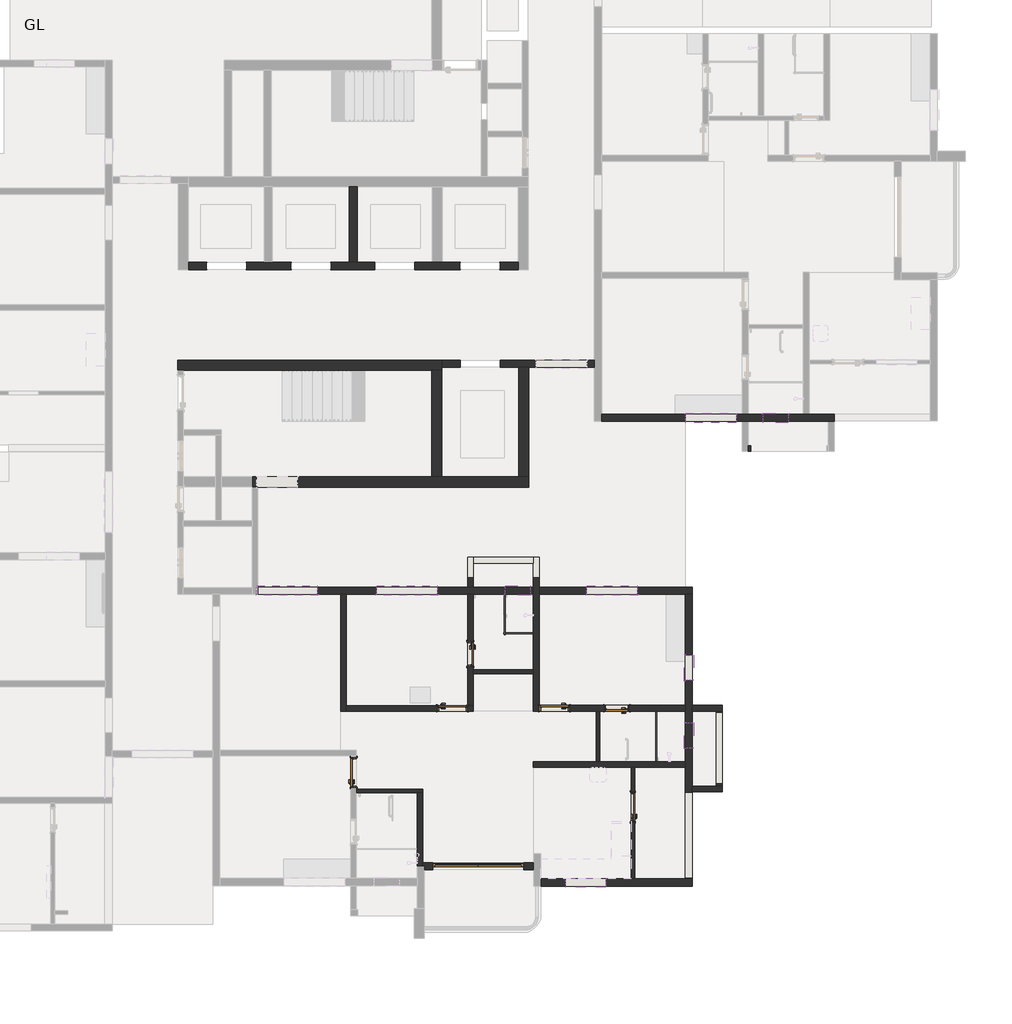
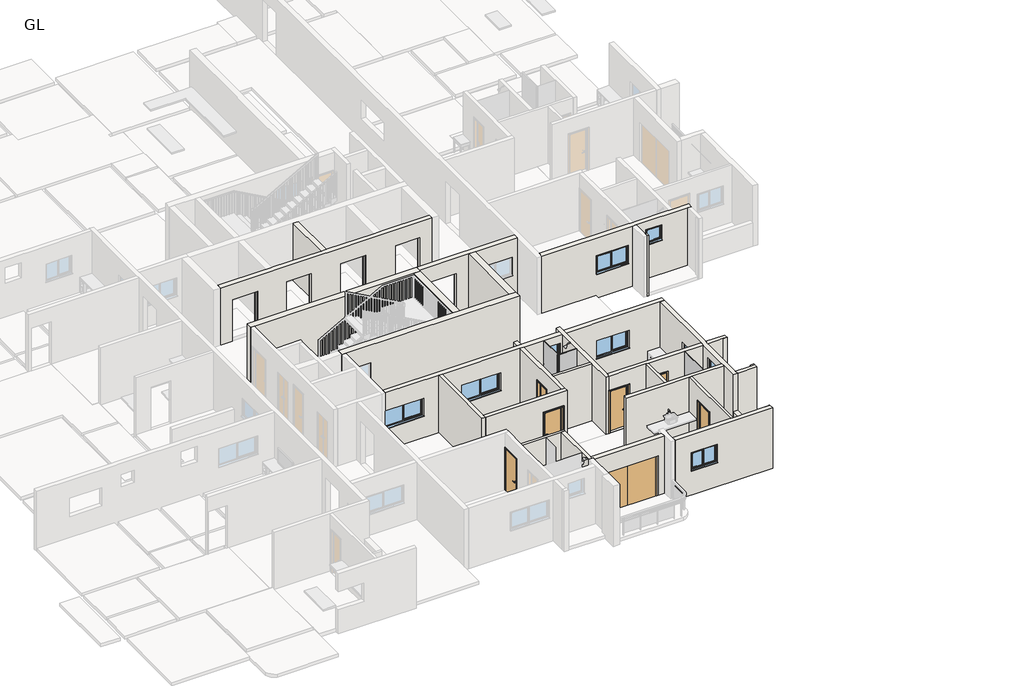
# One storey, part 4 of 14: 35 walls, 9 windows, 7 doors, 3 plates.
# Revit data of these elements (continued)
# Type "Windows_Dbl_Plain : 5'" (continued)
#   Rough Width = 5.0 ft
#   Rough Height = 2.985564 ft
#   Height = 2.985564 ft
#   Width = 5.0 ft
#   Heat Transfer Coefficient (U) = 3.6886 W/(m²·K)
#   Glazing Thickness = 0.07874 ft
#   FrameOffset - External = 0.164042 ft
#   Frame Depth = 0.213255 ft
#   Default Head Height = 6.922572 ft
#   Cill Depth = 0.287073 ft
#   Cavity Closer Width = 0.164042 ft
#   Cavity Closer Offset from Ext = 0.336286 ft
#   Cavity Closer Depth = 0.278871 ft
#   Vis - Cavity Closers = yes
#   Define Thermal Properties by = 1
#   Material Trim = Window Frame
#   Material Glass = Glass
#   Material Frame = Window Frame
#   Wall Closure = (empty or 0)
# Type "Windows_Dbl_Plain : 6'"
#   Type Mark = "62"
#   Operation = "DoublePanelVertical"
#   Construction Type Id = "GSP4R"
#   Manufacturer = "Revit"
#   Keynote = "L10"
#   Analytic Construction = "1/8 in Pilkington single glazing"
#   Wrap Layers (Ext) from Ext = 0.336286 ft
#   Wrap Layers (Int) from Ext = 0.582349 ft
#   Window Board Projection = 0.082021 ft
#   Window Board Extension = 0.082021 ft
#   Visual Light Transmittance = 0.9
#   Solar Heat Gain Coefficient = 0.78
#   Rough Width = 6.0 ft
#   Rough Height = 2.985564 ft
#   Height = 2.985564 ft
#   Width = 6.0 ft
#   Heat Transfer Coefficient (U) = 3.6886 W/(m²·K)
#   Glazing Thickness = 0.07874 ft
#   FrameOffset - External = 0.164042 ft
#   Frame Depth = 0.213255 ft
#   Default Head Height = 6.922572 ft
#   Cill Depth = 0.287073 ft
#   Cavity Closer Width = 0.164042 ft
#   Cavity Closer Offset from Ext = 0.336286 ft
#   Cavity Closer Depth = 0.278871 ft
#   Vis - Cavity Closers = yes
#   Define Thermal Properties by = 1
#   Material Trim = Window Frame
#   Material Glass = Glass
#   Material Frame = Window Frame
#   Wall Closure = (empty or 0)
# Type "Windows_Sgl_Plain : 2.5'"
#   Type Mark = "61"
#   Operation = "SinglePanel"
#   Construction Type Id = "SGL"
#   Manufacturer = "Revit"
#   Keynote = "L10"
#   Analytic Construction = "Large single-glazed windows"
#   Wrap Layers (Ext) from Ext = 0.336286 ft
#   Wrap Layers (Int) from Ext = 0.582349 ft
#   Window Board Projection = 0.082021 ft
#   Window Board Extension = 0.082021 ft
#   Visual Light Transmittance = 0.9
#   Solar Heat Gain Coefficient = 0.86
#   Rough Width = 2.5 ft
#   Rough Height = 2.5 ft
#   Height = 2.5 ft
#   Width = 2.5 ft
#   Heat Transfer Coefficient (U) = 5.5617 W/(m²·K)
#   Glazing Thickness = 0.07874 ft
#   FrameOffset - External = 0.164042 ft
#   Frame Depth = 0.213255 ft
#   Default Head Height = 6.922572 ft
#   Cill Depth = 0.287073 ft
#   Cavity Closer Width = 0.164042 ft
#   Cavity Closer Offset from Ext = 0.336286 ft
#   Cavity Closer Depth = 0.278871 ft
#   Vis - Cavity Closers = yes
#   Define Thermal Properties by = 1
#   Material Trim = Window Frame
#   Material Glass = Glass
#   Material Frame = Window Frame
#   Wall Closure = (empty or 0)
# Element 1 (IfcDoor, "Doors_Concept_ExtDbl : 9'")
#   Phase Created = New Construction
#   Materials on its faces: "Concept", "Door - Glazing"
# Elements 2, 3 (IfcDoor, "Doors_IntSgl : 2.5' DOOR")
#   Phase Created = New Construction
#   Materials on its faces: "Door - Architrave", "Door - Handle", "Door - Frame/Mullion (1)", "Door - Panel"
# Elements 4, 5, 6, 7 (IfcDoor, "Doors_IntSgl : 3' DOOR")
#   Phase Created = New Construction
#   Materials on its faces: "Door - Architrave", "Door - Handle", "Door - Frame/Mullion (1)", "Door - Panel"
# Elements 8, 9, 10 (IfcPlate, "System Panel : Glazed")
#   Phase Created = New Construction
#   Materials on its faces: "Glass"
# Elements 11, 12, 13, 14, 15, 16, 17, 21, 22, 23, 25, 26, 27 (IfcWall, "W2")
#   Top Offset = 0.0 ft
#   Base Offset = 0.0 ft
#   wall height = 9.84252 ft
#   Phase Created = New Construction
#   Base Constraint = GL
#   Top Constraint = FFL
#   Materials on its faces: "Brick, Common"
# Elements 18, 19, 20 (IfcWall, "W2")
#   Top Offset = -8.0 ft
#   Base Offset = 0.0 ft
#   wall height = 1.84252 ft
#   Phase Created = New Construction
#   Base Constraint = GL
#   Top Constraint = FFL
#   Materials on its faces: "Brick, Common"
# Element 24 (IfcWall, "W2")
#   Top Offset = -6.0 ft
#   Base Offset = 0.0 ft
#   wall height = 3.84252 ft
#   Phase Created = New Construction
#   Base Constraint = GL
#   Top Constraint = FFL
#   Materials on its faces: "Brick, Common"
# Elements 28, 29, 30, 31 (IfcWall, "W3")
#   Top Offset = 0.0 ft
#   Base Offset = 0.0 ft
#   wall height = 9.84252 ft
#   Phase Created = New Construction
#   Base Constraint = GL
#   Top Constraint = FFL
#   Materials on its faces: "Brick, Common"
# Elements 32, 33, 34, 35 (IfcWall, "W4")
#   Top Offset = 0.0 ft
#   Base Offset = 0.0 ft
#   wall height = 9.84252 ft
#   Phase Created = New Construction
#   Base Constraint = GL
#   Top Constraint = FFL
#   Materials on its faces: "Brick, Common"
# Element 36 (IfcWall, "W6")
#   Top Offset = 0.0 ft
#   Base Offset = 0.0 ft
#   wall height = 9.84252 ft
#   Phase Created = New Construction
#   Base Constraint = GL
#   Top Constraint = FFL
#   Materials on its faces: "Brick, Common"
# Elements 37, 38 (IfcWall, "W7")
#   Top Offset = 0.0 ft
#   Base Offset = 0.0 ft
#   wall height = 9.84252 ft
#   Phase Created = New Construction
#   Base Constraint = GL
#   Top Constraint = FFL
#   Materials on its faces: "Brick, Common"
# Elements 39, 40, 41, 42, 43, 45 (IfcWall, "W8")
#   Top Offset = 0.0 ft
#   Base Offset = 0.0 ft
#   wall height = 9.84252 ft
#   Phase Created = New Construction
#   Base Constraint = GL
#   Top Constraint = FFL
#   Materials on its faces: "Brick, Common"
# Element 44 (IfcWall, "W8")
#   Top Offset = -6.0 ft
#   Base Offset = 0.0 ft
#   wall height = 3.84252 ft
#   Phase Created = New Construction
#   Base Constraint = GL
#   Top Constraint = FFL
#   Materials on its faces: "Brick, Common"
# Element 46 (IfcWindow, "Windows_Dbl_Plain : 2.5'")
#   Mark = "19"
#   Phase Created = New Construction
#   Materials on its faces: "Window Frame", "Glass"
# Element 47 (IfcWindow, "Windows_Dbl_Plain : 4'")
#   Mark = "17"
#   Phase Created = New Construction
#   Materials on its faces: "Window Frame", "Glass"
# Element 48 (IfcWindow, "Windows_Dbl_Plain : 5'")
#   Mark = "20"
#   Phase Created = New Construction
#   Materials on its faces: "Window Frame", "Glass"
# Element 49 (IfcWindow, "Windows_Dbl_Plain : 5'")
#   Mark = "27"
#   Phase Created = New Construction
#   Materials on its faces: "Window Frame", "Glass"
# Element 50 (IfcWindow, "Windows_Dbl_Plain : 6'")
#   Mark = "22"
#   Phase Created = New Construction
#   Materials on its faces: "Window Frame", "Glass"
# Element 51 (IfcWindow, "Windows_Dbl_Plain : 6'")
#   Mark = "23"
#   Phase Created = New Construction
#   Materials on its faces: "Window Frame", "Glass"
# Element 52 (IfcWindow, "Windows_Sgl_Plain : 2.5'")
#   Mark = "18"
#   Phase Created = New Construction
#   Materials on its faces: "Window Frame", "Glass"
# Element 53 (IfcWindow, "Windows_Sgl_Plain : 2.5'")
#   Mark = "21"
#   Phase Created = New Construction
#   Materials on its faces: "Window Frame", "Glass"
# Element 54 (IfcWindow, "Windows_Sgl_Plain : 2.5'")
#   Mark = "28"
#   Phase Created = New Construction
#   Materials on its faces: "Window Frame", "Glass"
# Materials
#   "Door - Glazing": colour RGB 0 0 255, transparency 0.75
#   "Concept": colour RGB 128 128 255, transparency 0.5
#   "Door - Handle": colour RGB 0 0 0, transparency 0, Keynote = "P21", Cost = 0
#   "Door - Frame/Mullion (1)": class "Wood", colour RGB 212 179 113, transparency 0, Keynote = "L20", Cost = 0
#   "Door - Panel": class "Wood", colour RGB 210 159 95, transparency 0, Keynote = "L20", Cost = 0
#   "Door - Architrave": class "Wood", colour RGB 154 90 5, transparency 0, Keynote = "P20", Cost = 0
#   "Brick, Common": class "Masonry", colour RGB 170 100 105, transparency 0, Description = "Common brick", Cost = 0
#   "Window Frame": colour RGB 249 249 249, transparency 0, Keynote = "L10", Cost = 0
#   "Glass": class "Glass", colour RGB 0 128 192, transparency 0.9, Description = "Soda Lime Glass", Cost = 0
